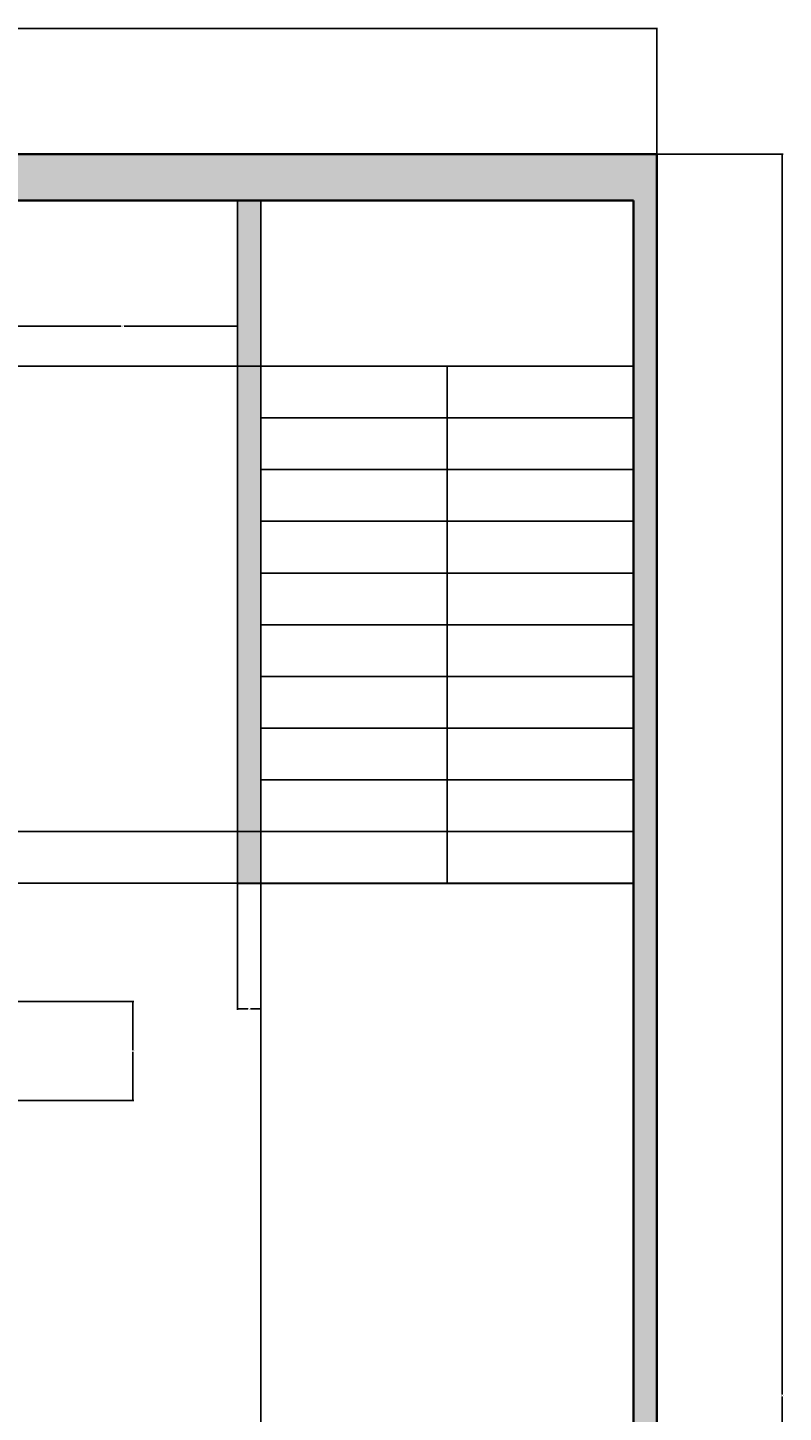
# Model space of a CAD drawing. Units: millimetres. Extents: x 2817 to 5038, y 1110 to 3565.
# Tile 19 of 21: x 3065 to 3211, y 1371 to 1639. Entities that reach past the tile are written whole.
import ezdxf

# ---------------------------------------------------------------- set-up
doc = ezdxf.new("R2010")
doc.units = ezdxf.units.MM
for name, color, linetype, lineweight in [('A-ANNO-DIMS', 2, 'Continuous', 18), ('A-FLOR-STRS', 7, 'Continuous', 25), ('A-WALL', 7, 'Continuous', 35)]:
    doc.layers.add(name, color=color, linetype=linetype, lineweight=lineweight)
doc.layers.add('A-WALL-PATT', color=51, linetype='Continuous', lineweight=13, true_color=0xf7f281)
doc.styles.get("Standard").update_dxf_attribs({"font": 'arial.ttf'})
doc.dimstyles.get("Standard").update_dxf_attribs({"dimtxt": 0.18, "dimasz": 0.18, "dimexe": 0.18, "dimexo": 0.0625, "dimgap": 0.09, "dimtad": 0, "dimtih": 1, "dimtoh": 1, "dimdec": 4, "dimzin": 0, "dimdsep": 46, "dimtxsty": 'Standard', "dimcen": 0.09, "dimadec": 0, "dimazin": 0, "dimtfac": 1, "dimtdec": 4, "dimtofl": 0, "dimtmove": 0, "dimatfit": 3, "dimfxl": 1, "dimtolj": 1, "dimtzin": 0, "dimarcsym": 0})

# ---------------------------------------------------------------- blocks, each defined once
blk = doc.blocks.new('*D26')
at = {"layer": 'A-ANNO-DIMS', "color": 0, "lineweight": -2, "transparency": 16777216}
for p, q in [((2841.74, 1614.5), (2841.74, 1638.87)), ((2841.92, 1638.69), (3013.95, 1638.69)), ((3186.56, 1638.69), (3014.53, 1638.69)), ((3186.74, 1614.5), (3186.74, 1638.87))]:
    blk.add_line(p, q, dxfattribs=at)
for points in [[(2841.92, 1638.72), (2841.92, 1638.66), (2841.74, 1638.69)], [(3186.56, 1638.72), (3186.56, 1638.66), (3186.74, 1638.69)]]:
    blk.add_solid(points, dxfattribs=at)
at = {"layer": 'Defpoints', "color": 0, "lineweight": -2, "transparency": 16777216}
for p in [(3186.74, 1638.69), (2841.74, 1614.44), (3186.74, 1614.44)]:
    blk.add_point(p, dxfattribs=at)
at = {"layer": 'A-ANNO-DIMS', "color": 0, "transparency": 16777216, "insert": (3014.24, 1638.69), "char_height": 0.18, "attachment_point": 5}
blk.add_mtext('\\A1;345', dxfattribs=at)
blk = doc.blocks.new('*D27')
at = {"layer": 'A-ANNO-DIMS', "color": 0, "lineweight": -2, "transparency": 16777216}
for p, q in [((3186.8, 1614.44), (3211.17, 1614.44)), ((3210.99, 1614.26), (3210.99, 1374.62)), ((3210.99, 1134.62), (3210.99, 1374.25)), ((3186.8, 1134.44), (3211.17, 1134.44))]:
    blk.add_line(p, q, dxfattribs=at)
for points in [[(3210.96, 1614.26), (3211.02, 1614.26), (3210.99, 1614.44)], [(3210.96, 1134.62), (3211.02, 1134.62), (3210.99, 1134.44)]]:
    blk.add_solid(points, dxfattribs=at)
at = {"layer": 'Defpoints', "color": 0, "lineweight": -2, "transparency": 16777216}
for p in [(3186.74, 1614.44), (3210.99, 1614.44), (3186.74, 1134.44)]:
    blk.add_point(p, dxfattribs=at)
at = {"layer": 'A-ANNO-DIMS', "color": 0, "transparency": 16777216, "insert": (3210.99, 1374.44), "char_height": 0.18, "attachment_point": 5}
blk.add_mtext('\\A1;480', dxfattribs=at)
blk = doc.blocks.new('*D37')
at = {"layer": 'A-ANNO-DIMS', "color": 0, "lineweight": -2, "transparency": 16777216}
for p, q in [((3110.24, 1473.37), (3110.24, 1110.01)), ((3182.24, 1473.37), (3182.24, 1110.01)), ((3110.42, 1110.19), (3146.02, 1110.19)), ((3182.06, 1110.19), (3146.46, 1110.19))]:
    blk.add_line(p, q, dxfattribs=at)
for points in [[(3110.42, 1110.22), (3110.42, 1110.16), (3110.24, 1110.19)], [(3182.06, 1110.22), (3182.06, 1110.16), (3182.24, 1110.19)]]:
    blk.add_solid(points, dxfattribs=at)
at = {"layer": 'Defpoints', "color": 0, "lineweight": -2, "transparency": 16777216}
for p in [(3110.24, 1473.44), (3182.24, 1473.44), (3182.24, 1110.19)]:
    blk.add_point(p, dxfattribs=at)
at = {"layer": 'A-ANNO-DIMS', "color": 0, "transparency": 16777216, "insert": (3146.24, 1110.19), "char_height": 0.18, "attachment_point": 5}
blk.add_mtext('\\A1;72', dxfattribs=at)
blk = doc.blocks.new('*D38')
at = {"layer": 'A-ANNO-DIMS', "color": 0, "lineweight": -2, "transparency": 16777216}
for p, q in [((3110.18, 1573.44), (2817.31, 1573.44)), ((2817.49, 1573.26), (2817.49, 1523.62)), ((2817.49, 1473.62), (2817.49, 1523.25)), ((3105.68, 1473.44), (2817.31, 1473.44))]:
    blk.add_line(p, q, dxfattribs=at)
for points in [[(2817.46, 1573.26), (2817.52, 1573.26), (2817.49, 1573.44)], [(2817.46, 1473.62), (2817.52, 1473.62), (2817.49, 1473.44)]]:
    blk.add_solid(points, dxfattribs=at)
at = {"layer": 'Defpoints', "color": 0, "lineweight": -2, "transparency": 16777216}
for p in [(2817.49, 1573.44), (3110.24, 1573.44), (3105.74, 1473.44)]:
    blk.add_point(p, dxfattribs=at)
at = {"layer": 'A-ANNO-DIMS', "color": 0, "transparency": 16777216, "insert": (2817.49, 1523.44), "char_height": 0.18, "attachment_point": 5}
blk.add_mtext('\\A1;100', dxfattribs=at)
blk = doc.blocks.new('*D39')
at = {"layer": 'A-ANNO-DIMS', "color": 0, "lineweight": -2, "transparency": 16777216}
for p, q in [((3105.68, 1605.44), (2817.31, 1605.44)), ((2817.49, 1605.26), (2817.49, 1589.62)), ((2817.49, 1573.62), (2817.49, 1589.25)), ((3110.18, 1573.44), (2817.31, 1573.44))]:
    blk.add_line(p, q, dxfattribs=at)
for points in [[(2817.46, 1605.26), (2817.52, 1605.26), (2817.49, 1605.44)], [(2817.46, 1573.62), (2817.52, 1573.62), (2817.49, 1573.44)]]:
    blk.add_solid(points, dxfattribs=at)
at = {"layer": 'Defpoints', "color": 0, "lineweight": -2, "transparency": 16777216}
for p in [(2817.49, 1605.44), (3105.74, 1605.44), (3110.24, 1573.44)]:
    blk.add_point(p, dxfattribs=at)
at = {"layer": 'A-ANNO-DIMS', "color": 0, "transparency": 16777216, "insert": (2817.49, 1589.44), "char_height": 0.18, "attachment_point": 5}
blk.add_mtext('\\A1;32', dxfattribs=at)
blk = doc.blocks.new('*D40')
at = {"layer": 'A-ANNO-DIMS', "color": 0, "lineweight": -2, "transparency": 16777216}
for p, q in [((3182.18, 1483.44), (2817.31, 1483.44)), ((2817.49, 1483.26), (2817.49, 1478.62)), ((2817.49, 1473.62), (2817.49, 1478.25)), ((3182.18, 1473.44), (2817.31, 1473.44))]:
    blk.add_line(p, q, dxfattribs=at)
for points in [[(2817.46, 1483.26), (2817.52, 1483.26), (2817.49, 1483.44)], [(2817.46, 1473.62), (2817.52, 1473.62), (2817.49, 1473.44)]]:
    blk.add_solid(points, dxfattribs=at)
at = {"layer": 'Defpoints', "color": 0, "lineweight": -2, "transparency": 16777216}
for p in [(2817.49, 1483.44), (3182.24, 1483.44), (3182.24, 1473.44)]:
    blk.add_point(p, dxfattribs=at)
at = {"layer": 'A-ANNO-DIMS', "color": 0, "transparency": 16777216, "insert": (2817.49, 1478.44), "char_height": 0.18, "attachment_point": 5}
blk.add_mtext('\\A1;10', dxfattribs=at)
blk = doc.blocks.new('*D41')
at = {"layer": 'A-ANNO-DIMS', "color": 0, "lineweight": -2, "transparency": 16777216}
for p, q in [((3061.24, 1605.37), (3061.24, 1581.01)), ((3105.74, 1605.37), (3105.74, 1581.01)), ((3061.42, 1581.19), (3083.16, 1581.19)), ((3105.56, 1581.19), (3083.82, 1581.19))]:
    blk.add_line(p, q, dxfattribs=at)
for points in [[(3061.42, 1581.22), (3061.42, 1581.16), (3061.24, 1581.19)], [(3105.56, 1581.22), (3105.56, 1581.16), (3105.74, 1581.19)]]:
    blk.add_solid(points, dxfattribs=at)
at = {"layer": 'Defpoints', "color": 0, "lineweight": -2, "transparency": 16777216}
for p in [(3061.24, 1605.44), (3105.74, 1605.44), (3061.24, 1581.19)]:
    blk.add_point(p, dxfattribs=at)
at = {"layer": 'A-ANNO-DIMS', "color": 0, "transparency": 16777216, "insert": (3083.49, 1581.19), "char_height": 0.18, "attachment_point": 5}
blk.add_mtext('\\A1;44.5', dxfattribs=at)
blk = doc.blocks.new('*D42')
at = {"layer": 'A-ANNO-DIMS', "color": 0, "lineweight": -2, "transparency": 16777216}
for p, q in [((3105.74, 1473.37), (3105.74, 1449.01)), ((3110.24, 1473.37), (3110.24, 1449.01)), ((3105.92, 1449.19), (3107.73, 1449.19)), ((3110.06, 1449.19), (3108.25, 1449.19))]:
    blk.add_line(p, q, dxfattribs=at)
for points in [[(3105.92, 1449.22), (3105.92, 1449.16), (3105.74, 1449.19)], [(3110.06, 1449.22), (3110.06, 1449.16), (3110.24, 1449.19)]]:
    blk.add_solid(points, dxfattribs=at)
at = {"layer": 'Defpoints', "color": 0, "lineweight": -2, "transparency": 16777216}
for p in [(3105.74, 1473.44), (3110.24, 1473.44), (3105.74, 1449.19)]:
    blk.add_point(p, dxfattribs=at)
at = {"layer": 'A-ANNO-DIMS', "color": 0, "transparency": 16777216, "insert": (3107.99, 1449.19), "char_height": 0.18, "attachment_point": 5}
blk.add_mtext('\\A1;4.5', dxfattribs=at)
blk = doc.blocks.new('*D49')
at = {"layer": 'A-ANNO-DIMS', "color": 0, "lineweight": -2, "transparency": 16777216}
for p, q in [((3061.3, 1450.61), (3085.67, 1450.61)), ((3085.49, 1450.43), (3085.49, 1441.21)), ((3085.49, 1431.62), (3085.49, 1440.84)), ((3061.3, 1431.44), (3085.67, 1431.44))]:
    blk.add_line(p, q, dxfattribs=at)
for points in [[(3085.46, 1450.43), (3085.52, 1450.43), (3085.49, 1450.61)], [(3085.46, 1431.62), (3085.52, 1431.62), (3085.49, 1431.44)]]:
    blk.add_solid(points, dxfattribs=at)
at = {"layer": 'Defpoints', "color": 0, "lineweight": -2, "transparency": 16777216}
for p in [(3061.24, 1450.61), (3061.24, 1431.44), (3085.49, 1431.44)]:
    blk.add_point(p, dxfattribs=at)
at = {"layer": 'A-ANNO-DIMS', "color": 0, "transparency": 16777216, "insert": (3085.49, 1441.02), "char_height": 0.18, "attachment_point": 5}
blk.add_mtext('\\A1;19.177', dxfattribs=at)

msp = doc.modelspace()

# ---------------------------------------------------------------- hatches: boundary and pattern name
at = {"layer": 'A-WALL-PATT'}
h = msp.add_hatch(color=256, dxfattribs=at)
h.dxf.hatch_style = 1
h.paths.add_polyline_path([(3186.7393, 1614.4357), (2841.7393, 1614.4357), (2841.7393, 1568.614), (2850.7393, 1568.7609), (2850.7393, 1605.4357), (2982.7393, 1605.4357), (2991.7393, 1605.4357), (3052.2393, 1605.4357), (3052.2393, 1573.7835), (3061.2393, 1573.7835), (3061.2393, 1605.4357), (3182.2393, 1605.4357), (3182.2393, 1143.4357), (3181.2393, 1143.4357), (3181.2393, 1134.4357), (3186.7393, 1134.4357)])
h.paths.add_polyline_path([(3061.2393, 1143.4357), (3061.2393, 1147.4357), (3052.2393, 1147.4357), (3052.2393, 1143.4357), (2850.7393, 1143.4357), (2850.7393, 1145.2996), (2841.7393, 1145.2996), (2841.7393, 1134.4357), (3061.2393, 1134.4357)], flags=17)
h.paths.add_polyline_path([(2850.7393, 1265.4357), (2946.7393, 1265.4357), (2946.7393, 1270.8357), (2946.7393, 1274.4357), (2850.7393, 1274.4357), (2850.7381, 1274.4357), (2850.7381, 1274.2564), (2841.7393, 1274.2564), (2841.7393, 1193.1527), (2850.7393, 1193.2996)], flags=17)
h.paths.add_polyline_path([(3061.2393, 1299.098), (3052.2393, 1299.098), (3052.2393, 1274.4357), (2991.7393, 1274.4357), (2991.7393, 1340.4357), (2982.7393, 1340.4357), (2982.7393, 1274.4357), (2982.7393, 1265.4357), (3052.2393, 1265.4357), (3052.2393, 1259.143), (3061.2393, 1259.2899)], flags=17)
h.paths.add_polyline_path([(3061.2393, 1383.4357), (3052.2393, 1383.4357), (3052.2393, 1379.4357), (2931.7393, 1379.4357), (2922.7393, 1379.4357), (2850.7393, 1379.4357), (2850.7381, 1379.4357), (2850.7381, 1379.3646), (2841.7393, 1379.3646), (2841.7393, 1322.1095), (2850.7393, 1322.2564), (2850.7393, 1370.4357), (2982.7393, 1370.4357), (2987.2393, 1370.4357), (3017.2393, 1370.4357), (3052.2393, 1370.4357), (3052.2393, 1323.098), (3061.2393, 1323.098)], flags=17)
h = msp.add_hatch(color=256, dxfattribs=at)
h.dxf.hatch_style = 1
h.paths.add_polyline_path([(3110.2393, 1605.4357), (3105.7393, 1605.4357), (3105.7393, 1473.4357), (3110.2393, 1473.4357)])

# ---------------------------------------------------------------- linework, layer by layer
at = {"layer": 'A-FLOR-STRS'}
for p, q in [((3105.7393, 1605.4357), (3105.7393, 1473.4357)), ((3110.2393, 1605.4357), (3110.2393, 1473.4357)), ((3110.2393, 1573.4357), (3182.2393, 1573.4357)), ((3146.2393, 1473.4357), (3146.2393, 1573.4357)), ((3110.2393, 1563.4357), (3182.2393, 1563.4357)), ((3110.2393, 1553.4357), (3182.2393, 1553.4357)), ((3110.2393, 1543.4357), (3182.2393, 1543.4357)), ((3110.2393, 1533.4357), (3182.2393, 1533.4357)), ((3110.2393, 1523.4357), (3182.2393, 1523.4357)), ((3110.2393, 1513.4357), (3182.2393, 1513.4357)), ((3110.2393, 1503.4357), (3182.2393, 1503.4357)), ((3110.2393, 1493.4357), (3182.2393, 1493.4357)), ((3110.2393, 1483.4357), (3182.2393, 1483.4357)), ((3105.7393, 1473.4357), (3182.2393, 1473.4357))]:
    msp.add_line(p, q, dxfattribs=at)
at = {"layer": 'A-WALL'}
for p, q in [((2841.7393, 1614.4357), (3186.7393, 1614.4357)), ((3186.7393, 1614.4357), (3186.7393, 1134.4357)), ((3061.2393, 1605.4357), (3182.2393, 1605.4357)), ((3182.2393, 1605.4357), (3182.2393, 1509.4357)), ((3182.2393, 1605.4357), (3182.2393, 1143.4357))]:
    msp.add_line(p, q, dxfattribs=at)

# ---------------------------------------------------------------- dimensions: what is measured, and where the dimension line sits
at = {"layer": 'A-ANNO-DIMS'}
for base, p1, p2, picture, middle in [((3186.7393, 1638.6857), (2841.7393, 1614.4357), (3186.7393, 1614.4357), '*D26', (3014.2393, 1638.6857)), ((3182.2393, 1110.1857), (3110.2393, 1473.4357), (3182.2393, 1473.4357), '*D37', (3146.2393, 1110.1857))]:
    dim = msp.add_linear_dim(base=base, p1=p1, p2=p2, dimstyle='Standard', override={"dimdec": 0, "dimlfac": 1, "dimrnd": 0, "dimzin": 0, "dimdsep": 46, "dimlunit": 2}, dxfattribs=at)
    dim.commit()
    dim.dimension.update_dxf_attribs({"geometry": picture, "text_midpoint": middle})
for base, p1, p2, angle, override, picture, middle in [((3210.9893, 1614.4357), (3186.7393, 1134.4357), (3186.7393, 1614.4357), 90, {"dimdec": 0, "dimlfac": 1, "dimrnd": 0, "dimzin": 0, "dimdsep": 46, "dimlunit": 2}, '*D27', (3210.9893, 1374.4357)), ((2817.4881, 1605.4357), (3110.2393, 1573.4357), (3105.7393, 1605.4357), 90, {"dimdec": 0, "dimlfac": 1, "dimrnd": 0, "dimzin": 0, "dimdsep": 46, "dimlunit": 2}, '*D39', (2817.4881, 1589.4357)), ((3061.2393, 1581.1857), (3105.7393, 1605.4357), (3061.2393, 1605.4357), 180, {"dimdec": 1, "dimlfac": 1, "dimrnd": 0, "dimzin": 0, "dimdsep": 46, "dimlunit": 2}, '*D41', (3083.4893, 1581.1857)), ((2817.4881, 1573.4357), (3105.7393, 1473.4357), (3110.2393, 1573.4357), 90, {"dimdec": 0, "dimlfac": 1, "dimrnd": 0, "dimzin": 0, "dimdsep": 46, "dimlunit": 2}, '*D38', (2817.4881, 1523.4357)), ((2817.4881, 1483.4357), (3182.2393, 1473.4357), (3182.2393, 1483.4357), 90, {"dimdec": 0, "dimlfac": 1, "dimrnd": 0, "dimzin": 0, "dimdsep": 46, "dimlunit": 2}, '*D40', (2817.4881, 1478.4357)), ((3105.7393, 1449.1857), (3110.2393, 1473.4357), (3105.7393, 1473.4357), 180, {"dimdec": 1, "dimlfac": 1, "dimrnd": 0, "dimzin": 0, "dimdsep": 46, "dimlunit": 2}, '*D42', (3107.9893, 1449.1857)), ((3085.4893, 1431.4357), (3061.2393, 1450.613), (3061.2393, 1431.4357), 270, {"dimdec": 3, "dimlfac": 1, "dimrnd": 0, "dimzin": 0, "dimdsep": 46, "dimlunit": 2}, '*D49', (3085.4893, 1441.0244))]:
    dim = msp.add_linear_dim(base=base, p1=p1, p2=p2, angle=angle, dimstyle='Standard', override=override, dxfattribs=at)
    dim.commit()
    dim.dimension.update_dxf_attribs({"geometry": picture, "text_midpoint": middle})

doc.saveas('drawing.dxf')
